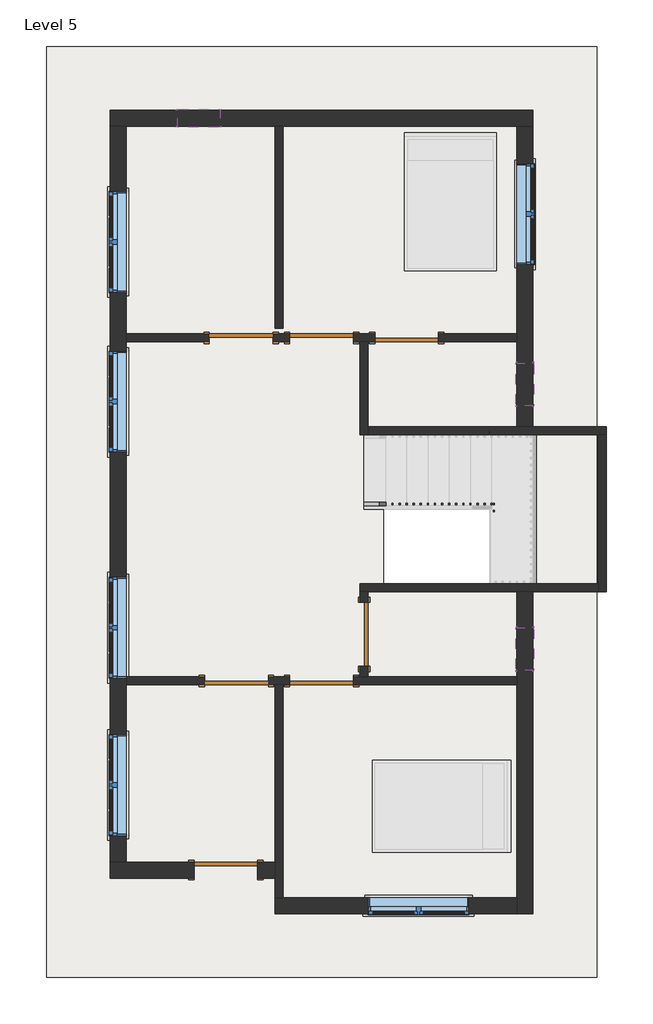
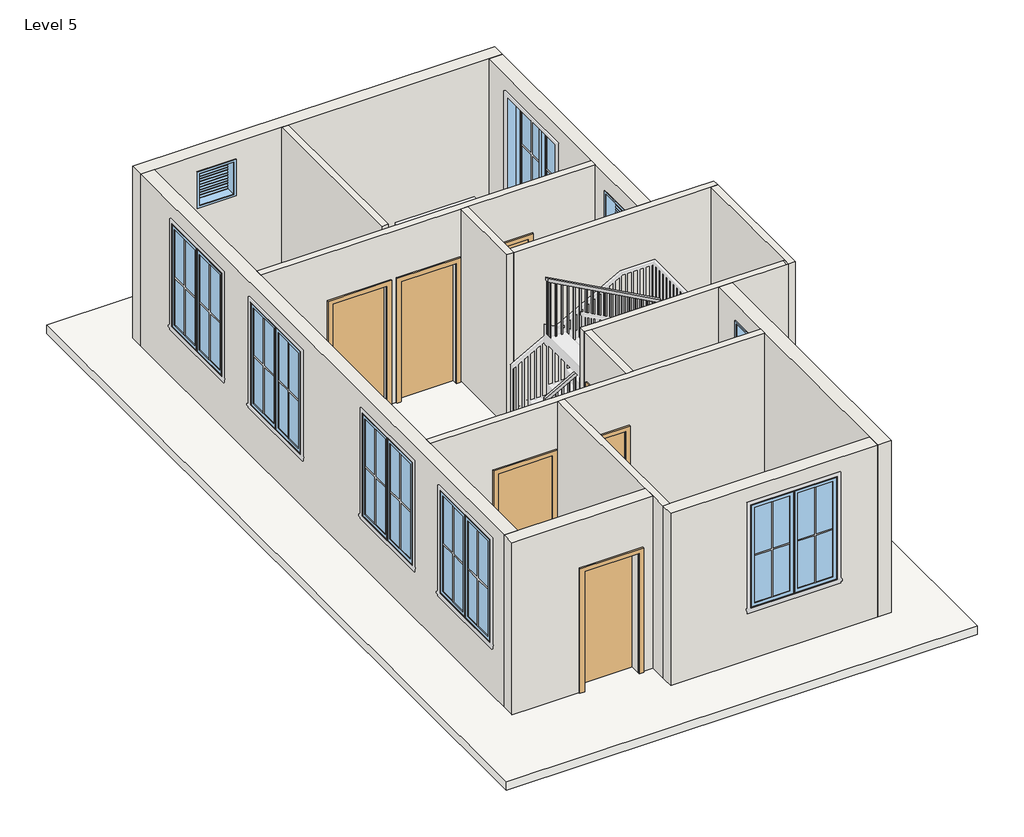
# One storey, part 1 of 2: 15 walls, 9 windows, 7 doors, 1 railing, 1 roof.
"""IFC4 building model written with IfcOpenShell, lengths in millimetres."""

from ifc_helpers import new_model, si_unit, frame, origin, place, context, project, spatial, polyline, outline, extrude, faceted_brep, transform, mapped, element, save
from components import door_e5f9f3c4, door_305aa2a5, door_0ca8825f, window_9ac97e1a, window_f2d8fef0

model = new_model("IFC4")

# Units and contexts
model_context = context("Model", 3, world=origin())
ifc_project = project(units=[si_unit("LENGTHUNIT", "METRE", prefix="MILLI")], contexts=[model_context])

# Site, building, storey
site = spatial("IfcSite", under=ifc_project)
building = spatial("IfcBuilding", under=site)
storey = spatial("IfcBuildingStorey", under=building, Name="Level 5", Elevation=9601.2)

# Doors
placement = place(None, origin())
door_shape = door_e5f9f3c4(model_context)
element("IfcDoor", 1, ObjectType="Single-Flush : 36\" x 84\"", at=placement, inside=storey, context=model_context, shape_type="MappedRepresentation", body=[
    mapped(door_shape, transform((-2929.7888307, 2238.9017201, 9601.2), x_axis=(1.0, 0.0, 0.0), y_axis=(0.0, 1.0, 0.0), z_axis=(0.0, 0.0, 1.0))),
])
element("IfcDoor", 2, ObjectType="Single-Flush : 36\" x 84\"", at=placement, inside=storey, context=model_context, shape_type="MappedRepresentation", body=[
    mapped(door_shape, transform((-558.0638307, 2238.9017201, 9601.2), x_axis=(-1.0, 0.0, 0.0), y_axis=(0.0, -1.0, 0.0), z_axis=(0.0, 0.0, 1.0))),
])
element("IfcDoor", 3, ObjectType="Single-Flush : 36\" x 84\"", at=placement, inside=storey, context=model_context, shape_type="MappedRepresentation", body=[
    mapped(door_shape, transform((-1167.6638307, -2009.2482799, 9601.2), x_axis=(0.0, -1.0, 0.0), y_axis=(1.0, 0.0, 0.0), z_axis=(0.0, 0.0, 1.0))),
])
element("IfcDoor", 4, ObjectType="Single-Flush : 36\" x 84\"", at=placement, inside=storey, context=model_context, shape_type="MappedRepresentation", body=[
    mapped(door_shape, transform((-1777.2638307, -2675.9982799, 9601.2), x_axis=(-1.0, 0.0, 0.0), y_axis=(0.0, -1.0, 0.0), z_axis=(0.0, 0.0, 1.0))),
])
door_2_shape = door_305aa2a5(model_context)
element("IfcDoor", 5, ObjectType="Single-Flush : 36\" x 84\"", at=placement, inside=storey, context=model_context, shape_type="MappedRepresentation", body=[
    mapped(door_2_shape, transform((-1777.2638307, 2238.9017201, 9601.2), x_axis=(-1.0, 0.0, 0.0), y_axis=(0.0, -1.0, 0.0), z_axis=(0.0, 0.0, 1.0))),
])
element("IfcDoor", 6, ObjectType="Single-Flush : 36\" x 84\"", at=placement, inside=storey, context=model_context, shape_type="MappedRepresentation", body=[
    mapped(door_2_shape, transform((-2996.4638307, -2675.9982799, 9601.2), x_axis=(1.0, 0.0, 0.0), y_axis=(0.0, 1.0, 0.0), z_axis=(0.0, 0.0, 1.0))),
])
door_3_shape = door_0ca8825f(model_context)
element("IfcDoor", 7, ObjectType="Single-Flush : 36\" x 84\"", at=placement, inside=storey, context=model_context, shape_type="MappedRepresentation", body=[
    mapped(door_3_shape, transform((-3148.8638307, -5387.4482799, 9601.2), x_axis=(1.0, 0.0, 0.0), y_axis=(0.0, 1.0, 0.0), z_axis=(0.0, 0.0, 1.0))),
])

# Railing
element("IfcRailing", 8, ObjectType="Handrail - Rectangular", at=placement, inside=storey, context=model_context, shape_type="SolidModel", body=[
    faceted_brep([(-1167.6638307, -116.9482799, 10684.9333333), (-1167.6638307, -116.9482799, 10626.8675836), (-1167.6638307, -167.7482799, 10626.8675836), (-1167.6638307, -167.7482799, 10684.9333333), (591.2861693, -116.9482799, 11658.7464821), (642.0861693, -116.9482799, 11628.8052998), (642.0861693, -167.7482799, 11628.8052998), (591.2861693, -167.7482799, 11658.7464821), (591.2861693, -116.9482799, 11700.9333333), (642.0861693, -116.9482799, 11650.1333333), (642.0861693, -167.7482799, 11650.1333333), (591.2861693, -167.7482799, 11700.9333333), (718.2861693, -116.9482799, 11700.9333333), (718.2861693, -116.9482799, 11650.1333333), (667.4861693, -167.7482799, 11650.1333333), (667.4861693, -167.7482799, 11700.9333333), (718.2861693, -218.5482799, 11700.9333333), (667.4861693, -218.5482799, 11700.9333333), (667.4861693, -269.3482799, 11650.1333333), (718.2861693, -269.3482799, 11650.1333333)], [[[0, 1, 2, 3]], [[1, 0, 4, 5]], [[2, 1, 5, 6]], [[3, 2, 6, 7]], [[0, 3, 7, 4]], [[5, 4, 8, 9]], [[6, 5, 9, 10]], [[7, 6, 10, 11]], [[4, 7, 11, 8]], [[9, 8, 12, 13]], [[10, 9, 13, 14]], [[11, 10, 14, 15]], [[8, 11, 15, 12]], [[16, 17, 18, 19]], [[13, 12, 16, 19]], [[14, 13, 19, 18]], [[15, 14, 18, 17]], [[12, 15, 17, 16]]]),
    faceted_brep([(718.2861693, -218.5482799, 11700.9333333), (718.2861693, -269.3482799, 11650.1333333), (667.4861693, -269.3482799, 11650.1333333), (667.4861693, -218.5482799, 11700.9333333), (718.2861693, -218.5482799, 11842.4310502), (667.4861693, -218.5482799, 11812.3403208), (667.4861693, -269.3482799, 11812.3403208), (718.2861693, -269.3482799, 11842.4310502)], [[[0, 1, 2, 3]], [[4, 5, 6, 7]], [[1, 0, 4, 7]], [[2, 1, 7, 6]], [[3, 2, 6, 5]], [[0, 3, 5, 4]]]),
    faceted_brep([(718.2861693, -269.3482799, 11842.4310502), (667.4861693, -269.3482799, 11812.3403208), (667.4861693, -218.5482799, 11812.3403208), (718.2861693, -218.5482799, 11842.4310502), (-1186.7138307, -269.3482799, 12886.2666667), (-1186.7138307, -218.5482799, 12886.2666667), (-1186.7138307, -218.5482799, 12828.3403208), (-1186.7138307, -269.3482799, 12828.3403208)], [[[0, 1, 2, 3]], [[4, 5, 6, 7]], [[1, 0, 4, 7]], [[2, 1, 7, 6]], [[3, 2, 6, 5]], [[0, 3, 5, 4]]]),
    extrude(outline(polyline([(12795.2855263, -1126.3888307), (12805.7238825, -1145.4388307), (11802.5333333, -1145.4388307), (11802.5333333, -1126.3888307), (12795.2855263, -1126.3888307)])), frame((0.0, -253.4732799, 0.0), z_axis=(0.0, 1.0, 0.0), x_axis=(0.0, 0.0, 1.0)), (0.0, 0.0, 1.0), 19.05),
    extrude(outline(polyline([(12739.6142934, -1024.7888307), (12750.0526496, -1043.8388307), (11802.5333333, -1043.8388307), (11802.5333333, -1024.7888307), (12739.6142934, -1024.7888307)])), frame((0.0, -253.4732799, 0.0), z_axis=(0.0, 1.0, 0.0), x_axis=(0.0, 0.0, 1.0)), (0.0, 0.0, 1.0), 19.05),
    extrude(outline(polyline([(12683.9430606, -923.1888307), (12694.3814167, -942.2388307), (11802.5333333, -942.2388307), (11802.5333333, -923.1888307), (12683.9430606, -923.1888307)])), frame((0.0, -253.4732799, 0.0), z_axis=(0.0, 1.0, 0.0), x_axis=(0.0, 0.0, 1.0)), (0.0, 0.0, 1.0), 19.05),
    extrude(outline(polyline([(12628.2718277, -821.5888307), (12638.7101838, -840.6388307), (11633.2, -840.6388307), (11633.2, -821.5888307), (12628.2718277, -821.5888307)])), frame((0.0, -253.4732799, 0.0), z_axis=(0.0, 1.0, 0.0), x_axis=(0.0, 0.0, 1.0)), (0.0, 0.0, 1.0), 19.05),
    extrude(outline(polyline([(12572.6005948, -719.9888307), (12583.038951, -739.0388307), (11633.2, -739.0388307), (11633.2, -719.9888307), (12572.6005948, -719.9888307)])), frame((0.0, -253.4732799, 0.0), z_axis=(0.0, 1.0, 0.0), x_axis=(0.0, 0.0, 1.0)), (0.0, 0.0, 1.0), 19.05),
    extrude(outline(polyline([(12516.9293619, -618.3888307), (12527.3677181, -637.4388307), (11633.2, -637.4388307), (11633.2, -618.3888307), (12516.9293619, -618.3888307)])), frame((0.0, -253.4732799, 0.0), z_axis=(0.0, 1.0, 0.0), x_axis=(0.0, 0.0, 1.0)), (0.0, 0.0, 1.0), 19.05),
    extrude(outline(polyline([(12461.258129, -516.7888307), (12471.6964852, -535.8388307), (11463.8666667, -535.8388307), (11463.8666667, -516.7888307), (12461.258129, -516.7888307)])), frame((0.0, -253.4732799, 0.0), z_axis=(0.0, 1.0, 0.0), x_axis=(0.0, 0.0, 1.0)), (0.0, 0.0, 1.0), 19.05),
    extrude(outline(polyline([(12405.5868962, -415.1888307), (12416.0252523, -434.2388307), (11463.8666667, -434.2388307), (11463.8666667, -415.1888307), (12405.5868962, -415.1888307)])), frame((0.0, -253.4732799, 0.0), z_axis=(0.0, 1.0, 0.0), x_axis=(0.0, 0.0, 1.0)), (0.0, 0.0, 1.0), 19.05),
    extrude(outline(polyline([(12349.9156633, -313.5888307), (12360.3540195, -332.6388307), (11463.8666667, -332.6388307), (11463.8666667, -313.5888307), (12349.9156633, -313.5888307)])), frame((0.0, -253.4732799, 0.0), z_axis=(0.0, 1.0, 0.0), x_axis=(0.0, 0.0, 1.0)), (0.0, 0.0, 1.0), 19.05),
    extrude(outline(polyline([(12294.2444304, -211.9888307), (12304.6827866, -231.0388307), (11294.5333333, -231.0388307), (11294.5333333, -211.9888307), (12294.2444304, -211.9888307)])), frame((0.0, -253.4732799, 0.0), z_axis=(0.0, 1.0, 0.0), x_axis=(0.0, 0.0, 1.0)), (0.0, 0.0, 1.0), 19.05),
    extrude(outline(polyline([(12238.5731975, -110.3888307), (12249.0115537, -129.4388307), (11294.5333333, -129.4388307), (11294.5333333, -110.3888307), (12238.5731975, -110.3888307)])), frame((0.0, -253.4732799, 0.0), z_axis=(0.0, 1.0, 0.0), x_axis=(0.0, 0.0, 1.0)), (0.0, 0.0, 1.0), 19.05),
    extrude(outline(polyline([(12182.9019647, -8.7888307), (12193.3403208, -27.8388307), (11294.5333333, -27.8388307), (11294.5333333, -8.7888307), (12182.9019647, -8.7888307)])), frame((0.0, -253.4732799, 0.0), z_axis=(0.0, 1.0, 0.0), x_axis=(0.0, 0.0, 1.0)), (0.0, 0.0, 1.0), 19.05),
    extrude(outline(polyline([(12127.2307318, 92.8111693), (12137.6690879, 73.7611693), (11125.2, 73.7611693), (11125.2, 92.8111693), (12127.2307318, 92.8111693)])), frame((0.0, -253.4732799, 0.0), z_axis=(0.0, 1.0, 0.0), x_axis=(0.0, 0.0, 1.0)), (0.0, 0.0, 1.0), 19.05),
    extrude(outline(polyline([(12071.5594989, 194.4111693), (12081.9978551, 175.3611693), (11125.2, 175.3611693), (11125.2, 194.4111693), (12071.5594989, 194.4111693)])), frame((0.0, -253.4732799, 0.0), z_axis=(0.0, 1.0, 0.0), x_axis=(0.0, 0.0, 1.0)), (0.0, 0.0, 1.0), 19.05),
    extrude(outline(polyline([(12015.888266, 296.0111693), (12026.3266222, 276.9611693), (11125.2, 276.9611693), (11125.2, 296.0111693), (12015.888266, 296.0111693)])), frame((0.0, -253.4732799, 0.0), z_axis=(0.0, 1.0, 0.0), x_axis=(0.0, 0.0, 1.0)), (0.0, 0.0, 1.0), 19.05),
    extrude(outline(polyline([(11960.2170332, 397.6111693), (11970.6553893, 378.5611693), (10955.8666667, 378.5611693), (10955.8666667, 397.6111693), (11960.2170332, 397.6111693)])), frame((0.0, -253.4732799, 0.0), z_axis=(0.0, 1.0, 0.0), x_axis=(0.0, 0.0, 1.0)), (0.0, 0.0, 1.0), 19.05),
    extrude(outline(polyline([(11904.5458003, 499.2111693), (11914.9841564, 480.1611693), (10955.8666667, 480.1611693), (10955.8666667, 499.2111693), (11904.5458003, 499.2111693)])), frame((0.0, -253.4732799, 0.0), z_axis=(0.0, 1.0, 0.0), x_axis=(0.0, 0.0, 1.0)), (0.0, 0.0, 1.0), 19.05),
    extrude(outline(polyline([(11848.8745674, 600.8111693), (11859.3129236, 581.7611693), (10955.8666667, 581.7611693), (10955.8666667, 600.8111693), (11848.8745674, 600.8111693)])), frame((0.0, -253.4732799, 0.0), z_axis=(0.0, 1.0, 0.0), x_axis=(0.0, 0.0, 1.0)), (0.0, 0.0, 1.0), 19.05),
    extrude(outline(polyline([(651.6111693, -151.8732799), (651.6111693, -132.8232799), (670.6611693, -132.8232799), (670.6611693, -151.8732799), (651.6111693, -151.8732799)])), frame((0.0, 0.0, 10617.2), z_axis=(0.0, 0.0, 1.0), x_axis=(1.0, 0.0, 0.0)), (0.0, 0.0, 1.0), 1032.9333333),
    extrude(outline(polyline([(11588.3762341, 569.0611693), (11577.8295213, 550.0111693), (10617.2, 550.0111693), (10617.2, 569.0611693), (11588.3762341, 569.0611693)])), frame((0.0, -151.8732799, 0.0), z_axis=(0.0, 1.0, 0.0), x_axis=(0.0, 0.0, 1.0)), (0.0, 0.0, 1.0), 19.05),
    extrude(outline(polyline([(11532.1270991, 467.4611693), (11521.5803863, 448.4111693), (10617.2, 448.4111693), (10617.2, 467.4611693), (11532.1270991, 467.4611693)])), frame((0.0, -151.8732799, 0.0), z_axis=(0.0, 1.0, 0.0), x_axis=(0.0, 0.0, 1.0)), (0.0, 0.0, 1.0), 19.05),
    extrude(outline(polyline([(11475.8779642, 365.8611693), (11465.3312514, 346.8111693), (10447.8666667, 346.8111693), (10447.8666667, 365.8611693), (11475.8779642, 365.8611693)])), frame((0.0, -151.8732799, 0.0), z_axis=(0.0, 1.0, 0.0), x_axis=(0.0, 0.0, 1.0)), (0.0, 0.0, 1.0), 19.05),
    extrude(outline(polyline([(11419.6288292, 264.2611693), (11409.0821164, 245.2111693), (10447.8666667, 245.2111693), (10447.8666667, 264.2611693), (11419.6288292, 264.2611693)])), frame((0.0, -151.8732799, 0.0), z_axis=(0.0, 1.0, 0.0), x_axis=(0.0, 0.0, 1.0)), (0.0, 0.0, 1.0), 19.05),
    extrude(outline(polyline([(11363.3796943, 162.6611693), (11352.8329815, 143.6111693), (10447.8666667, 143.6111693), (10447.8666667, 162.6611693), (11363.3796943, 162.6611693)])), frame((0.0, -151.8732799, 0.0), z_axis=(0.0, 1.0, 0.0), x_axis=(0.0, 0.0, 1.0)), (0.0, 0.0, 1.0), 19.05),
    extrude(outline(polyline([(11307.1305593, 61.0611693), (11296.5838465, 42.0111693), (10278.5333333, 42.0111693), (10278.5333333, 61.0611693), (11307.1305593, 61.0611693)])), frame((0.0, -151.8732799, 0.0), z_axis=(0.0, 1.0, 0.0), x_axis=(0.0, 0.0, 1.0)), (0.0, 0.0, 1.0), 19.05),
    extrude(outline(polyline([(11250.8814244, -40.5388307), (11240.3347116, -59.5888307), (10278.5333333, -59.5888307), (10278.5333333, -40.5388307), (11250.8814244, -40.5388307)])), frame((0.0, -151.8732799, 0.0), z_axis=(0.0, 1.0, 0.0), x_axis=(0.0, 0.0, 1.0)), (0.0, 0.0, 1.0), 19.05),
    extrude(outline(polyline([(11194.6322895, -142.1388307), (11184.0855766, -161.1888307), (10278.5333333, -161.1888307), (10278.5333333, -142.1388307), (11194.6322895, -142.1388307)])), frame((0.0, -151.8732799, 0.0), z_axis=(0.0, 1.0, 0.0), x_axis=(0.0, 0.0, 1.0)), (0.0, 0.0, 1.0), 19.05),
    extrude(outline(polyline([(11138.3831545, -243.7388307), (11127.8364417, -262.7888307), (10109.2, -262.7888307), (10109.2, -243.7388307), (11138.3831545, -243.7388307)])), frame((0.0, -151.8732799, 0.0), z_axis=(0.0, 1.0, 0.0), x_axis=(0.0, 0.0, 1.0)), (0.0, 0.0, 1.0), 19.05),
    extrude(outline(polyline([(11082.1340196, -345.3388307), (11071.5873068, -364.3888307), (10109.2, -364.3888307), (10109.2, -345.3388307), (11082.1340196, -345.3388307)])), frame((0.0, -151.8732799, 0.0), z_axis=(0.0, 1.0, 0.0), x_axis=(0.0, 0.0, 1.0)), (0.0, 0.0, 1.0), 19.05),
    extrude(outline(polyline([(11025.8848846, -446.9388307), (11015.3381718, -465.9888307), (10109.2, -465.9888307), (10109.2, -446.9388307), (11025.8848846, -446.9388307)])), frame((0.0, -151.8732799, 0.0), z_axis=(0.0, 1.0, 0.0), x_axis=(0.0, 0.0, 1.0)), (0.0, 0.0, 1.0), 19.05),
    extrude(outline(polyline([(10969.6357497, -548.5388307), (10959.0890369, -567.5888307), (9939.8666667, -567.5888307), (9939.8666667, -548.5388307), (10969.6357497, -548.5388307)])), frame((0.0, -151.8732799, 0.0), z_axis=(0.0, 1.0, 0.0), x_axis=(0.0, 0.0, 1.0)), (0.0, 0.0, 1.0), 19.05),
    extrude(outline(polyline([(10913.3866147, -650.1388307), (10902.8399019, -669.1888307), (9939.8666667, -669.1888307), (9939.8666667, -650.1388307), (10913.3866147, -650.1388307)])), frame((0.0, -151.8732799, 0.0), z_axis=(0.0, 1.0, 0.0), x_axis=(0.0, 0.0, 1.0)), (0.0, 0.0, 1.0), 19.05),
    extrude(outline(polyline([(10857.1374798, -751.7388307), (10846.590767, -770.7888307), (9939.8666667, -770.7888307), (9939.8666667, -751.7388307), (10857.1374798, -751.7388307)])), frame((0.0, -151.8732799, 0.0), z_axis=(0.0, 1.0, 0.0), x_axis=(0.0, 0.0, 1.0)), (0.0, 0.0, 1.0), 19.05),
    extrude(outline(polyline([(10800.8883448, -853.3388307), (10790.341632, -872.3888307), (9770.5333333, -872.3888307), (9770.5333333, -853.3388307), (10800.8883448, -853.3388307)])), frame((0.0, -151.8732799, 0.0), z_axis=(0.0, 1.0, 0.0), x_axis=(0.0, 0.0, 1.0)), (0.0, 0.0, 1.0), 19.05),
    extrude(outline(polyline([(10744.6392099, -954.9388307), (10734.0924971, -973.9888307), (9770.5333333, -973.9888307), (9770.5333333, -954.9388307), (10744.6392099, -954.9388307)])), frame((0.0, -151.8732799, 0.0), z_axis=(0.0, 1.0, 0.0), x_axis=(0.0, 0.0, 1.0)), (0.0, 0.0, 1.0), 19.05),
    extrude(outline(polyline([(10688.3900749, -1056.5388307), (10677.8433621, -1075.5888307), (9770.5333333, -1075.5888307), (9770.5333333, -1056.5388307), (10688.3900749, -1056.5388307)])), frame((0.0, -151.8732799, 0.0), z_axis=(0.0, 1.0, 0.0), x_axis=(0.0, 0.0, 1.0)), (0.0, 0.0, 1.0), 19.05),
    extrude(outline(polyline([(683.3611693, -234.4232799), (702.4111693, -234.4232799), (702.4111693, -253.4732799), (683.3611693, -253.4732799), (683.3611693, -234.4232799)])), frame((0.0, 0.0, 10786.5333333), z_axis=(0.0, 0.0, 1.0), x_axis=(1.0, 0.0, 0.0)), (0.0, 0.0, 1.0), 863.6),
    extrude(outline(polyline([(683.3611693, -151.8732799), (683.3611693, -132.8232799), (702.4111693, -132.8232799), (702.4111693, -151.8732799), (683.3611693, -151.8732799)])), frame((0.0, 0.0, 10786.5333333), z_axis=(0.0, 0.0, 1.0), x_axis=(1.0, 0.0, 0.0)), (0.0, 0.0, 1.0), 863.6),
    extrude(outline(polyline([(12817.9019647, -1167.6638307), (12828.3403208, -1186.7138307), (11802.5333333, -1186.7138307), (11802.5333333, -1167.6638307), (12817.9019647, -1167.6638307)])), frame((0.0, -253.4732799, 0.0), z_axis=(0.0, 1.0, 0.0), x_axis=(0.0, 0.0, 1.0)), (0.0, 0.0, 1.0), 19.05),
    extrude(outline(polyline([(10637.4142964, -1148.6138307), (10626.8675836, -1167.6638307), (9770.5333333, -1167.6638307), (9770.5333333, -1148.6138307), (10637.4142964, -1148.6138307)])), frame((0.0, -151.8732799, 0.0), z_axis=(0.0, 1.0, 0.0), x_axis=(0.0, 0.0, 1.0)), (0.0, 0.0, 1.0), 19.05),
])

# Roof
element("IfcRoof", 9, ObjectType="ROOF 6\"", at=placement, inside=storey, context=model_context, shape_type="SweptSolid", body=[
    extrude(outline(polyline([(-5720.6138307, -6924.1482799), (-5720.6138307, 6410.8517201), (2166.0861693, 6410.8517201), (2166.0861693, -6924.1482799), (-5720.6138307, -6924.1482799)]), holes=[polyline([(1251.6861693, -1285.3482799), (1251.6861693, 899.0517201), (-881.9138307, 899.0517201), (-881.9138307, -1285.3482799), (1251.6861693, -1285.3482799)])]), frame((0.0, 0.0, 9448.8), z_axis=(0.0, 0.0, 1.0), x_axis=(1.0, 0.0, 0.0)), (0.0, 0.0, 1.0), 152.4),
])

# Walls
element("IfcWall", 10, ObjectType="WALL 4.5\"", at=placement, inside=storey, context=model_context, shape_type="SweptSolid", body=[
    extrude(outline(polyline([(-2444.0138307, 2372.2517201), (-2444.0138307, 5267.8517201), (-2329.7138307, 5267.8517201), (-2329.7138307, 2372.2517201), (-2444.0138307, 2372.2517201)])), frame((0.0, 0.0, 9601.2), z_axis=(0.0, 0.0, 1.0), x_axis=(1.0, 0.0, 0.0)), (0.0, 0.0, 1.0), 3048.0),
])
element("IfcWall", 11, ObjectType="WALL 4.5\"", at=placement, inside=storey, context=model_context, shape_type="Brep", body=[
    faceted_brep([(-1320.0638307, 2181.7517201, 9601.2), (-1224.8138307, 2181.7517201, 9601.2), (-1110.5138307, 2181.7517201, 9601.2), (-1015.2638307, 2181.7517201, 9601.2), (-1015.2638307, 2181.7517201, 11734.8), (-100.8638307, 2181.7517201, 11734.8), (-100.8638307, 2181.7517201, 9601.2), (1023.0861693, 2181.7517201, 9601.2), (1023.0861693, 2181.7517201, 12649.2), (-1110.5138307, 2181.7517201, 12649.2), (-1224.8138307, 2181.7517201, 12649.2), (-4577.6138307, 2181.7517201, 12649.2), (-4577.6138307, 2181.7517201, 9601.2), (-3386.9888307, 2181.7517201, 9601.2), (-3386.9888307, 2181.7517201, 11734.8), (-2472.5888307, 2181.7517201, 11734.8), (-2472.5888307, 2181.7517201, 9601.2), (-2234.4638307, 2181.7517201, 9601.2), (-2234.4638307, 2181.7517201, 11734.8), (-1320.0638307, 2181.7517201, 11734.8), (-1015.2638307, 2296.0517201, 11734.8), (-1015.2638307, 2296.0517201, 9601.2), (-1320.0638307, 2296.0517201, 9601.2), (-1320.0638307, 2296.0517201, 11734.8), (-2234.4638307, 2296.0517201, 11734.8), (-2234.4638307, 2296.0517201, 9601.2), (-2472.5888307, 2296.0517201, 9601.2), (-2472.5888307, 2296.0517201, 11734.8), (-3386.9888307, 2296.0517201, 11734.8), (-3386.9888307, 2296.0517201, 9601.2), (-4577.6138307, 2296.0517201, 9601.2), (-4577.6138307, 2296.0517201, 12649.2), (1023.0861693, 2296.0517201, 12649.2), (1023.0861693, 2296.0517201, 9601.2), (-100.8638307, 2296.0517201, 9601.2), (-100.8638307, 2296.0517201, 11734.8)], [[[0, 1, 2, 3, 4, 5, 6, 7, 8, 9, 10, 11, 12, 13, 14, 15, 16, 17, 18, 19]], [[20, 21, 22, 23, 24, 25, 26, 27, 28, 29, 30, 31, 32, 33, 34, 35]], [[13, 12, 30, 29]], [[26, 25, 17, 16]], [[34, 33, 7, 6]], [[22, 21, 3, 2, 1, 0]], [[8, 7, 33, 32]], [[12, 11, 31, 30]], [[27, 26, 16, 15]], [[28, 27, 15, 14]], [[29, 28, 14, 13]], [[18, 17, 25, 24]], [[19, 18, 24, 23]], [[0, 19, 23, 22]], [[4, 3, 21, 20]], [[5, 4, 20, 35]], [[6, 5, 35, 34]], [[11, 10, 9, 8, 32, 31]]]),
])
element("IfcWall", 12, ObjectType="WALL 4.5\"", at=placement, inside=storey, context=model_context, shape_type="Brep", body=[
    faceted_brep([(-1224.8138307, 2181.7517201, 9601.2), (-1224.8138307, 848.2517201, 9601.2), (-1224.8138307, 848.2517201, 12649.2), (-1224.8138307, 2181.7517201, 12649.2), (-1110.5138307, 2181.7517201, 9601.2), (-1110.5138307, 2181.7517201, 12649.2), (-1110.5138307, 962.5517201, 12649.2), (-1110.5138307, 848.2517201, 12649.2), (-1110.5138307, 848.2517201, 9601.2), (-1110.5138307, 962.5517201, 9601.2)], [[[0, 1, 2, 3]], [[4, 5, 6, 7, 8, 9]], [[1, 0, 4, 9, 8]], [[0, 3, 5, 4]], [[2, 1, 8, 7]], [[3, 2, 7, 6, 5]]]),
])
element("IfcWall", 13, ObjectType="WALL 4.5\"", at=placement, inside=storey, context=model_context, shape_type="Brep", body=[
    faceted_brep([(-1110.5138307, 848.2517201, 9601.2), (2191.4861693, 848.2517201, 9601.2), (2305.7861693, 848.2517201, 9601.2), (2305.7861693, 848.2517201, 12649.2), (2191.4861693, 848.2517201, 12649.2), (-1110.5138307, 848.2517201, 12649.2), (-1110.5138307, 962.5517201, 9601.2), (-1110.5138307, 962.5517201, 12649.2), (1023.0861693, 962.5517201, 12649.2), (1251.6861693, 962.5517201, 12649.2), (2305.7861693, 962.5517201, 12649.2), (2305.7861693, 962.5517201, 9601.2), (1251.6861693, 962.5517201, 9601.2), (1023.0861693, 962.5517201, 9601.2)], [[[0, 1, 2, 3, 4, 5]], [[6, 7, 8, 9, 10, 11, 12, 13]], [[2, 1, 0, 6, 13, 12, 11]], [[5, 4, 3, 10, 9, 8, 7]], [[0, 5, 7, 6]], [[3, 2, 11, 10]]]),
])
element("IfcWall", 14, ObjectType="WALL 4.5\"", at=placement, inside=storey, context=model_context, shape_type="Brep", body=[
    faceted_brep([(2191.4861693, 848.2517201, 9601.2), (2191.4861693, -1285.3482799, 9601.2), (2191.4861693, -1399.6482799, 9601.2), (2191.4861693, -1399.6482799, 12649.2), (2191.4861693, -1285.3482799, 12649.2), (2191.4861693, 848.2517201, 12649.2), (2305.7861693, 848.2517201, 9601.2), (2305.7861693, 848.2517201, 12649.2), (2305.7861693, -1399.6482799, 12649.2), (2305.7861693, -1399.6482799, 9601.2)], [[[0, 1, 2, 3, 4, 5]], [[6, 7, 8, 9]], [[2, 1, 0, 6, 9]], [[5, 4, 3, 8, 7]], [[0, 5, 7, 6]], [[3, 2, 9, 8]]]),
])
element("IfcWall", 15, ObjectType="WALL 4.5\"", at=placement, inside=storey, context=model_context, shape_type="Brep", body=[
    faceted_brep([(2191.4861693, -1285.3482799, 9601.2), (-1224.8138307, -1285.3482799, 9601.2), (-1224.8138307, -1285.3482799, 12649.2), (-881.9138307, -1285.3482799, 12649.2), (1251.6861693, -1285.3482799, 12649.2), (2166.0861693, -1285.3482799, 12649.2), (2191.4861693, -1285.3482799, 12649.2), (2191.4861693, -1399.6482799, 9601.2), (2191.4861693, -1399.6482799, 12649.2), (2166.0861693, -1399.6482799, 12649.2), (1251.6861693, -1399.6482799, 12649.2), (1023.0861693, -1399.6482799, 12649.2), (-1110.5138307, -1399.6482799, 12649.2), (-1224.8138307, -1399.6482799, 12649.2), (-1224.8138307, -1399.6482799, 9601.2), (-1110.5138307, -1399.6482799, 9601.2), (1023.0861693, -1399.6482799, 9601.2), (1251.6861693, -1399.6482799, 9601.2)], [[[0, 1, 2, 3, 4, 5, 6]], [[7, 8, 9, 10, 11, 12, 13, 14, 15, 16, 17]], [[1, 0, 7, 17, 16, 15, 14]], [[0, 6, 8, 7]], [[2, 1, 14, 13]], [[6, 5, 9, 8]], [[5, 4, 3, 2, 13, 12, 11, 10, 9]]]),
])
element("IfcWall", 16, ObjectType="WALL 4.5\"", at=placement, inside=storey, context=model_context, shape_type="SweptSolid", body=[
    extrude(outline(polyline([(-2466.4482799, 11734.8), (-2466.4482799, 9601.2), (-2618.8482799, 9601.2), (-2618.8482799, 12649.2), (-1399.6482799, 12649.2), (-1399.6482799, 9601.2), (-1552.0482799, 9601.2), (-1552.0482799, 11734.8), (-2466.4482799, 11734.8)])), frame((-1224.8138307, 0.0, 0.0), z_axis=(1.0, 0.0, 0.0), x_axis=(0.0, 1.0, 0.0)), (0.0, 0.0, 1.0), 114.3),
])
element("IfcWall", 17, ObjectType="WALL 4.5\"", at=placement, inside=storey, context=model_context, shape_type="Brep", body=[
    faceted_brep([(-2234.4638307, -2618.8482799, 9601.2), (-2539.2638307, -2618.8482799, 9601.2), (-2539.2638307, -2618.8482799, 11734.8), (-3453.6638307, -2618.8482799, 11734.8), (-3453.6638307, -2618.8482799, 9601.2), (-4577.6138307, -2618.8482799, 9601.2), (-4577.6138307, -2618.8482799, 12649.2), (-1224.8138307, -2618.8482799, 12649.2), (-1110.5138307, -2618.8482799, 12649.2), (1023.0861693, -2618.8482799, 12649.2), (1023.0861693, -2618.8482799, 9601.2), (-1110.5138307, -2618.8482799, 9601.2), (-1224.8138307, -2618.8482799, 9601.2), (-1320.0638307, -2618.8482799, 9601.2), (-1320.0638307, -2618.8482799, 11734.8), (-2234.4638307, -2618.8482799, 11734.8), (-2539.2638307, -2733.1482799, 11734.8), (-2539.2638307, -2733.1482799, 9601.2), (-2444.0138307, -2733.1482799, 9601.2), (-2329.7138307, -2733.1482799, 9601.2), (-2234.4638307, -2733.1482799, 9601.2), (-2234.4638307, -2733.1482799, 11734.8), (-1320.0638307, -2733.1482799, 11734.8), (-1320.0638307, -2733.1482799, 9601.2), (1023.0861693, -2733.1482799, 9601.2), (1023.0861693, -2733.1482799, 12649.2), (-2329.7138307, -2733.1482799, 12649.2), (-2444.0138307, -2733.1482799, 12649.2), (-4577.6138307, -2733.1482799, 12649.2), (-4577.6138307, -2733.1482799, 9601.2), (-3453.6638307, -2733.1482799, 9601.2), (-3453.6638307, -2733.1482799, 11734.8)], [[[0, 1, 2, 3, 4, 5, 6, 7, 8, 9, 10, 11, 12, 13, 14, 15]], [[16, 17, 18, 19, 20, 21, 22, 23, 24, 25, 26, 27, 28, 29, 30, 31]], [[13, 12, 11, 10, 24, 23]], [[30, 29, 5, 4]], [[20, 19, 18, 17, 1, 0]], [[10, 9, 25, 24]], [[6, 5, 29, 28]], [[21, 20, 0, 15]], [[22, 21, 15, 14]], [[23, 22, 14, 13]], [[2, 1, 17, 16]], [[3, 2, 16, 31]], [[4, 3, 31, 30]], [[9, 8, 7, 6, 28, 27, 26, 25]]]),
])
element("IfcWall", 18, ObjectType="WALL 4.5\"", at=placement, inside=storey, context=model_context, shape_type="Brep", body=[
    faceted_brep([(-2329.7138307, -5781.1482799, 9601.2), (-2329.7138307, -2733.1482799, 9601.2), (-2329.7138307, -2733.1482799, 12649.2), (-2329.7138307, -5781.1482799, 12649.2), (-2444.0138307, -5781.1482799, 9601.2), (-2444.0138307, -5781.1482799, 12649.2), (-2444.0138307, -5501.7482799, 12649.2), (-2444.0138307, -5273.1482799, 12649.2), (-2444.0138307, -2733.1482799, 12649.2), (-2444.0138307, -2733.1482799, 9601.2), (-2444.0138307, -5273.1482799, 9601.2), (-2444.0138307, -5501.7482799, 9601.2)], [[[0, 1, 2, 3]], [[4, 5, 6, 7, 8, 9, 10, 11]], [[1, 0, 4, 11, 10, 9]], [[0, 3, 5, 4]], [[2, 1, 9, 8]], [[3, 2, 8, 7, 6, 5]]]),
])
element("IfcWall", 19, ObjectType="WALL 9\"", at=placement, inside=storey, context=model_context, shape_type="Brep", body=[
    faceted_brep([(-4806.2138307, 5267.8517201, 9601.2), (-4577.6138307, 5267.8517201, 9601.2), (-2444.0138307, 5267.8517201, 9601.2), (-2329.7138307, 5267.8517201, 9601.2), (1023.0861693, 5267.8517201, 9601.2), (1251.6861693, 5267.8517201, 9601.2), (1251.6861693, 5267.8517201, 12649.2), (1023.0861693, 5267.8517201, 12649.2), (-2329.7138307, 5267.8517201, 12649.2), (-2444.0138307, 5267.8517201, 12649.2), (-4577.6138307, 5267.8517201, 12649.2), (-4806.2138307, 5267.8517201, 12649.2), (-3844.1888307, 5267.8517201, 12344.4), (-3234.5888307, 5267.8517201, 12344.4), (-3234.5888307, 5267.8517201, 11734.8), (-3844.1888307, 5267.8517201, 11734.8), (-4806.2138307, 5496.4517201, 9601.2), (-4806.2138307, 5496.4517201, 12649.2), (1251.6861693, 5496.4517201, 12649.2), (1251.6861693, 5496.4517201, 9601.2), (-3844.1888307, 5496.4517201, 12344.4), (-3844.1888307, 5496.4517201, 11734.8), (-3234.5888307, 5496.4517201, 11734.8), (-3234.5888307, 5496.4517201, 12344.4)], [[[0, 1, 2, 3, 4, 5, 6, 7, 8, 9, 10, 11], [12, 13, 14, 15]], [[16, 17, 18, 19], [20, 21, 22, 23]], [[5, 4, 3, 2, 1, 0, 16, 19]], [[6, 5, 19, 18]], [[0, 11, 17, 16]], [[21, 20, 12, 15]], [[22, 21, 15, 14]], [[23, 22, 14, 13]], [[20, 23, 13, 12]], [[11, 10, 9, 8, 7, 6, 18, 17]]]),
])
element("IfcWall", 20, ObjectType="WALL 9\"", at=placement, inside=storey, context=model_context, shape_type="Brep", body=[
    faceted_brep([(1023.0861693, 5267.8517201, 9601.2), (1023.0861693, 2296.0517201, 9601.2), (1023.0861693, 2181.7517201, 9601.2), (1023.0861693, 962.5517201, 9601.2), (1023.0861693, 962.5517201, 12649.2), (1023.0861693, 2181.7517201, 12649.2), (1023.0861693, 2296.0517201, 12649.2), (1023.0861693, 5267.8517201, 12649.2), (1023.0861693, 3286.6517201, 12344.4), (1023.0861693, 3286.6517201, 10515.6), (1023.0861693, 4734.4517201, 10515.6), (1023.0861693, 4734.4517201, 12344.4), (1023.0861693, 1876.9517201, 12344.4), (1023.0861693, 1267.3517201, 12344.4), (1023.0861693, 1267.3517201, 11734.8), (1023.0861693, 1876.9517201, 11734.8), (1251.6861693, 5267.8517201, 9601.2), (1251.6861693, 5267.8517201, 12649.2), (1251.6861693, 962.5517201, 12649.2), (1251.6861693, 962.5517201, 9601.2), (1251.6861693, 3286.6517201, 12344.4), (1251.6861693, 4734.4517201, 12344.4), (1251.6861693, 4734.4517201, 10515.6), (1251.6861693, 3286.6517201, 10515.6), (1251.6861693, 1876.9517201, 12344.4), (1251.6861693, 1876.9517201, 11734.8), (1251.6861693, 1267.3517201, 11734.8), (1251.6861693, 1267.3517201, 12344.4)], [[[0, 1, 2, 3, 4, 5, 6, 7], [8, 9, 10, 11], [12, 13, 14, 15]], [[16, 17, 18, 19], [20, 21, 22, 23], [24, 25, 26, 27]], [[3, 2, 1, 0, 16, 19]], [[0, 7, 17, 16]], [[4, 3, 19, 18]], [[9, 8, 20, 23]], [[10, 9, 23, 22]], [[11, 10, 22, 21]], [[8, 11, 21, 20]], [[25, 24, 12, 15]], [[26, 25, 15, 14]], [[27, 26, 14, 13]], [[24, 27, 13, 12]], [[7, 6, 5, 4, 18, 17]]]),
])
element("IfcWall", 21, ObjectType="WALL 9\"", at=placement, inside=storey, context=model_context, shape_type="Brep", body=[
    faceted_brep([(1023.0861693, -1399.6482799, 9601.2), (1023.0861693, -2618.8482799, 9601.2), (1023.0861693, -2733.1482799, 9601.2), (1023.0861693, -5781.1482799, 9601.2), (1023.0861693, -6009.7482799, 9601.2), (1023.0861693, -6009.7482799, 12649.2), (1023.0861693, -5781.1482799, 12649.2), (1023.0861693, -2733.1482799, 12649.2), (1023.0861693, -2618.8482799, 12649.2), (1023.0861693, -1399.6482799, 12649.2), (1023.0861693, -1913.9982799, 12344.4), (1023.0861693, -2523.5982799, 12344.4), (1023.0861693, -2523.5982799, 11734.8), (1023.0861693, -1913.9982799, 11734.8), (1251.6861693, -1399.6482799, 9601.2), (1251.6861693, -1399.6482799, 12649.2), (1251.6861693, -6009.7482799, 12649.2), (1251.6861693, -6009.7482799, 9601.2), (1251.6861693, -1913.9982799, 12344.4), (1251.6861693, -1913.9982799, 11734.8), (1251.6861693, -2523.5982799, 11734.8), (1251.6861693, -2523.5982799, 12344.4)], [[[0, 1, 2, 3, 4, 5, 6, 7, 8, 9], [10, 11, 12, 13]], [[14, 15, 16, 17], [18, 19, 20, 21]], [[4, 3, 2, 1, 0, 14, 17]], [[5, 4, 17, 16]], [[0, 9, 15, 14]], [[19, 18, 10, 13]], [[20, 19, 13, 12]], [[21, 20, 12, 11]], [[18, 21, 11, 10]], [[9, 8, 7, 6, 5, 16, 15]]]),
])
element("IfcWall", 22, ObjectType="WALL 9\"", at=placement, inside=storey, context=model_context, shape_type="Brep", body=[
    faceted_brep([(1023.0861693, -5781.1482799, 9601.2), (-2329.7138307, -5781.1482799, 9601.2), (-2444.0138307, -5781.1482799, 9601.2), (-2444.0138307, -5781.1482799, 12649.2), (-2329.7138307, -5781.1482799, 12649.2), (1023.0861693, -5781.1482799, 12649.2), (-1110.5138307, -5781.1482799, 12344.4), (-1110.5138307, -5781.1482799, 10515.6), (337.2861693, -5781.1482799, 10515.6), (337.2861693, -5781.1482799, 12344.4), (1023.0861693, -6009.7482799, 9601.2), (1023.0861693, -6009.7482799, 12649.2), (-2444.0138307, -6009.7482799, 12649.2), (-2444.0138307, -6009.7482799, 9601.2), (-1110.5138307, -6009.7482799, 12344.4), (337.2861693, -6009.7482799, 12344.4), (337.2861693, -6009.7482799, 10515.6), (-1110.5138307, -6009.7482799, 10515.6)], [[[0, 1, 2, 3, 4, 5], [6, 7, 8, 9]], [[10, 11, 12, 13], [14, 15, 16, 17]], [[2, 1, 0, 10, 13]], [[0, 5, 11, 10]], [[3, 2, 13, 12]], [[7, 6, 14, 17]], [[8, 7, 17, 16]], [[9, 8, 16, 15]], [[6, 9, 15, 14]], [[5, 4, 3, 12, 11]]]),
])
element("IfcWall", 23, ObjectType="WALL 9\"", at=placement, inside=storey, context=model_context, shape_type="Brep", body=[
    faceted_brep([(-2691.6638307, -5501.7482799, 11734.8), (-2691.6638307, -5501.7482799, 9601.2), (-2444.0138307, -5501.7482799, 9601.2), (-2444.0138307, -5501.7482799, 12649.2), (-4806.2138307, -5501.7482799, 12649.2), (-4806.2138307, -5501.7482799, 9601.2), (-3606.0638307, -5501.7482799, 9601.2), (-3606.0638307, -5501.7482799, 11734.8), (-2444.0138307, -5273.1482799, 9601.2), (-2691.6638307, -5273.1482799, 9601.2), (-2691.6638307, -5273.1482799, 11734.8), (-3606.0638307, -5273.1482799, 11734.8), (-3606.0638307, -5273.1482799, 9601.2), (-4577.6138307, -5273.1482799, 9601.2), (-4806.2138307, -5273.1482799, 9601.2), (-4806.2138307, -5273.1482799, 12649.2), (-4577.6138307, -5273.1482799, 12649.2), (-2444.0138307, -5273.1482799, 12649.2)], [[[0, 1, 2, 3, 4, 5, 6, 7]], [[8, 9, 10, 11, 12, 13, 14, 15, 16, 17]], [[6, 5, 14, 13, 12]], [[2, 1, 9, 8]], [[5, 4, 15, 14]], [[3, 2, 8, 17]], [[10, 9, 1, 0]], [[11, 10, 0, 7]], [[12, 11, 7, 6]], [[4, 3, 17, 16, 15]]]),
])
element("IfcWall", 24, ObjectType="WALL 9\"", at=placement, inside=storey, context=model_context, shape_type="Brep", body=[
    faceted_brep([(-4577.6138307, -5273.1482799, 9601.2), (-4577.6138307, -2733.1482799, 9601.2), (-4577.6138307, -2618.8482799, 9601.2), (-4577.6138307, 2181.7517201, 9601.2), (-4577.6138307, 2296.0517201, 9601.2), (-4577.6138307, 5267.8517201, 9601.2), (-4577.6138307, 5267.8517201, 12649.2), (-4577.6138307, 2296.0517201, 12649.2), (-4577.6138307, 2181.7517201, 12649.2), (-4577.6138307, -2618.8482799, 12649.2), (-4577.6138307, -2733.1482799, 12649.2), (-4577.6138307, -5273.1482799, 12649.2), (-4577.6138307, -3444.3482799, 12344.4), (-4577.6138307, -3444.3482799, 10515.6), (-4577.6138307, -4892.1482799, 10515.6), (-4577.6138307, -4892.1482799, 12344.4), (-4577.6138307, -1190.0982799, 12344.4), (-4577.6138307, -1190.0982799, 10515.6), (-4577.6138307, -2637.8982799, 10515.6), (-4577.6138307, -2637.8982799, 12344.4), (-4577.6138307, 4334.4017201, 12344.4), (-4577.6138307, 4334.4017201, 10515.6), (-4577.6138307, 2886.6017201, 10515.6), (-4577.6138307, 2886.6017201, 12344.4), (-4577.6138307, 2048.4017201, 12344.4), (-4577.6138307, 2048.4017201, 10515.6), (-4577.6138307, 600.6017201, 10515.6), (-4577.6138307, 600.6017201, 12344.4), (-4806.2138307, -5273.1482799, 9601.2), (-4806.2138307, -5273.1482799, 12649.2), (-4806.2138307, 5267.8517201, 12649.2), (-4806.2138307, 5267.8517201, 9601.2), (-4806.2138307, -3444.3482799, 12344.4), (-4806.2138307, -4892.1482799, 12344.4), (-4806.2138307, -4892.1482799, 10515.6), (-4806.2138307, -3444.3482799, 10515.6), (-4806.2138307, -1190.0982799, 12344.4), (-4806.2138307, -2637.8982799, 12344.4), (-4806.2138307, -2637.8982799, 10515.6), (-4806.2138307, -1190.0982799, 10515.6), (-4806.2138307, 4334.4017201, 12344.4), (-4806.2138307, 2886.6017201, 12344.4), (-4806.2138307, 2886.6017201, 10515.6), (-4806.2138307, 4334.4017201, 10515.6), (-4806.2138307, 2048.4017201, 12344.4), (-4806.2138307, 600.6017201, 12344.4), (-4806.2138307, 600.6017201, 10515.6), (-4806.2138307, 2048.4017201, 10515.6)], [[[0, 1, 2, 3, 4, 5, 6, 7, 8, 9, 10, 11], [12, 13, 14, 15], [16, 17, 18, 19], [20, 21, 22, 23], [24, 25, 26, 27]], [[28, 29, 30, 31], [32, 33, 34, 35], [36, 37, 38, 39], [40, 41, 42, 43], [44, 45, 46, 47]], [[5, 4, 3, 2, 1, 0, 28, 31]], [[6, 5, 31, 30]], [[0, 11, 29, 28]], [[13, 12, 32, 35]], [[14, 13, 35, 34]], [[15, 14, 34, 33]], [[12, 15, 33, 32]], [[17, 16, 36, 39]], [[18, 17, 39, 38]], [[19, 18, 38, 37]], [[16, 19, 37, 36]], [[21, 20, 40, 43]], [[22, 21, 43, 42]], [[23, 22, 42, 41]], [[20, 23, 41, 40]], [[25, 24, 44, 47]], [[26, 25, 47, 46]], [[27, 26, 46, 45]], [[24, 27, 45, 44]], [[11, 10, 9, 8, 7, 6, 30, 29]]]),
])

# Windows
window_shape = window_9ac97e1a(model_context)
element("IfcWindow", 25, ObjectType="Window-Casement-Double : 57\" x 72\"", at=placement, inside=storey, context=model_context, shape_type="MappedRepresentation", body=[
    mapped(window_shape, transform((-4691.9138307, -4168.2482799, 9601.2), x_axis=(0.0, 1.0, 0.0), y_axis=(-1.0, 0.0, 0.0), z_axis=(0.0, 0.0, 1.0))),
])
element("IfcWindow", 26, ObjectType="Window-Casement-Double : 57\" x 72\"", at=placement, inside=storey, context=model_context, shape_type="MappedRepresentation", body=[
    mapped(window_shape, transform((-4691.9138307, -1913.9982799, 9601.2), x_axis=(0.0, 1.0, 0.0), y_axis=(-1.0, 0.0, 0.0), z_axis=(0.0, 0.0, 1.0))),
])
element("IfcWindow", 27, ObjectType="Window-Casement-Double : 57\" x 72\"", at=placement, inside=storey, context=model_context, shape_type="MappedRepresentation", body=[
    mapped(window_shape, transform((-386.6138307, -5895.4482799, 9601.2), x_axis=(-1.0, 0.0, 0.0), y_axis=(0.0, -1.0, 0.0), z_axis=(0.0, 0.0, 1.0))),
])
element("IfcWindow", 28, ObjectType="Window-Casement-Double : 57\" x 72\"", at=placement, inside=storey, context=model_context, shape_type="MappedRepresentation", body=[
    mapped(window_shape, transform((1137.3861693, 4010.5517201, 9601.2), x_axis=(0.0, -1.0, 0.0), y_axis=(1.0, 0.0, 0.0), z_axis=(0.0, 0.0, 1.0))),
])
element("IfcWindow", 29, ObjectType="Window-Casement-Double : 57\" x 72\"", at=placement, inside=storey, context=model_context, shape_type="MappedRepresentation", body=[
    mapped(window_shape, transform((-4691.9138307, 3610.5017201, 9601.2), x_axis=(0.0, 1.0, 0.0), y_axis=(-1.0, 0.0, 0.0), z_axis=(0.0, 0.0, 1.0))),
])
element("IfcWindow", 30, ObjectType="Window-Casement-Double : 57\" x 72\"", at=placement, inside=storey, context=model_context, shape_type="MappedRepresentation", body=[
    mapped(window_shape, transform((-4691.9138307, 1324.5017201, 9601.2), x_axis=(0.0, 1.0, 0.0), y_axis=(-1.0, 0.0, 0.0), z_axis=(0.0, 0.0, 1.0))),
])
window_2_shape = window_f2d8fef0(model_context)
element("IfcWindow", 31, ObjectType="Window-Louvers : 24\" x 24\"", at=placement, inside=storey, context=model_context, shape_type="MappedRepresentation", body=[
    mapped(window_2_shape, transform((1143.7361693, 1572.1517201, 10820.4), x_axis=(0.0, -1.0, 0.0), y_axis=(1.0, 0.0, 0.0), z_axis=(0.0, 0.0, 1.0))),
])
element("IfcWindow", 32, ObjectType="Window-Louvers : 24\" x 24\"", at=placement, inside=storey, context=model_context, shape_type="MappedRepresentation", body=[
    mapped(window_2_shape, transform((-3539.3888307, 5388.5017201, 10820.4), x_axis=(1.0, 0.0, 0.0), y_axis=(0.0, 1.0, 0.0), z_axis=(0.0, 0.0, 1.0))),
])
element("IfcWindow", 33, ObjectType="Window-Louvers : 24\" x 24\"", at=placement, inside=storey, context=model_context, shape_type="MappedRepresentation", body=[
    mapped(window_2_shape, transform((1143.7361693, -2218.7982799, 10820.4), x_axis=(0.0, -1.0, 0.0), y_axis=(1.0, 0.0, 0.0), z_axis=(0.0, 0.0, 1.0))),
])

save(model, "model.ifc")

# Revit data of these elements
# Type "Single-Flush : 36\" x 84\""
#   Type Mark = "1"
#   Construction Type Id = "MDOOR"
#   Assembly Code = "C1020"
#   Analytic Construction = "Metal"
#   Thickness = 0' - 2"
#   Heat Transfer Coefficient (U) = 0.651978 BTU/(h·ft²·°F)
#   Height = 7' - 0"
#   Trim Projection Ext = 0' - 1"
#   Trim Projection Int = 0' - 1"
#   Trim Width = 0' - 3"
#   Width = 3' - 0"
#   Define Thermal Properties by = 1
#   Define Thermal Properties by = 1
#   Door Material = Door - Panel
#   Frame Material = Door - Frame
#   Visual Light Transmittance = 0
#   Solar Heat Gain Coefficient = 0
#   Function = (empty or 0)
#   Wall Closure = (empty or 0)
# Type "Handrail - Rectangular"
#   Assembly Code = "C2010400"
#   built-in parameter 1008612 = 0.0416667 (stored number, unit not read)
#   built-in parameter 1008611 = 0.0416667 (stored number, unit not read)
#   built-in parameter 1008609 = 0.333333 (stored number, unit not read)
#   built-in parameter 1008604 = 0.166667 (stored number, unit not read)
#   built-in parameter 1008603 = 0.166667 (stored number, unit not read)
#   Railing Height = 3' - 0"
#   built-in parameter 1008630 = 2
#   built-in parameter 1008610 = 2
#   built-in parameter 1008618 = Baluster - Square : 3/4"
# Type "ROOF 6\""
#   Assembly Code = "B1020"
#   Layers, outside or top first: 0' - 6" no material (function 1)
# Type "WALL 4.5\""
#   Assembly Code = "B2010"
#   Layers, outside or top first: 0' - 4 1/2" no material (function 1)
# Type "WALL 9\""
#   Assembly Code = "B2010"
#   Layers, outside or top first: 0' - 9" no material (function 1)
# Type "Window-Casement-Double : 57\" x 72\""
#   Type Mark = "17"
#   Fire Rating = "0.5h"
#   Assembly Code = "B2020100"
#   Analytic Construction = "Double glazing - domestic"
#   Frame Extension [instance default] = 0' - 0 1/4"
#   Window Inset [instance default] = 0' - 0"
#   Wall Thickness [instance default] = 0' - 6"
#   Interior Wall Closure [instance default] = 0' - 2 1/4"
#   Half Width = 2' - 4 1/2"
#   Visual Light Transmittance = 0.81
#   Thermal Resistance (R) = 1.8146 (h·ft²·°F)/BTU
#   Solar Heat Gain Coefficient = 0.76
#   Rough Width = 4' - 9 1/2"
#   Rough Height = 6' - 0 1/2"
#   Height = 6' - 0"
#   Heat Transfer Coefficient (U) = 0.5511 BTU/(h·ft²·°F)
#   Exterior Wall Closure [instance default] = 0' - 1 1/4"
#   Extension Jamb [instance default] = 0' - 2 1/4"
#   Default Sill Height = 3' - 0"
#   Width = 4' - 9"
#   Define Thermal Properties by = 0
#   Muntin Visibility = yes
#   Interior Trim Visibility [instance default] = yes
#   Exterior Trim Visibility [instance default] = yes
#   Extension Jamb Visibility [instance default] = yes
#   Interior Trim Material = Wood - Stained
#   Muntin Pattern = Muntin Pattern_2x2 : Muntin Pattern_2x2
#   Interior Trim = Trim-Window-Interior-Flat : Picture Frame
#   Interior Frame Material = Wood - Stained
#   Glass Panel Material = Glass
#   Exterior Trim Material = Clad - White
#   Exterior Trim = Trim-Window-Exterior-Flat : with Sill
#   Exterior Frame Material = Clad - White
#   Wall Closure = (empty or 0)
# Type "Window-Louvers : 24\" x 24\""
#   Type Mark = "18"
#   Construction Type Id = "GSP4R"
#   Assembly Code = "B20"
#   Analytic Construction = "1/8 in Pilkington single glazing"
#   Visual Light Transmittance = 0.9
#   Thermal Resistance (R) = 1.53941 (h·ft²·°F)/BTU
#   Solar Heat Gain Coefficient = 0.78
#   Max Height = 1' - 11.74264"
#   Height = 2' - 0"
#   Heat Transfer Coefficient (U) = 0.6496 BTU/(h·ft²·°F)
#   Blade Width [instance default] = 1' - 10 1/2"
#   Blade Vertical Thickness = 0' - 0.35355"
#   Blade Thickness = 0' - 0 1/4"
#   Blade Spacing = 0' - 1 1/2"
#   Blade Height = 0' - 1.85355"
#   Blade Depth = 0' - 3"
#   Blade Angle = 45.00°
#   Default Sill Height = 3' - 0"
#   Trim Projection_Exterior = 0' - 0 1/2"
#   Trim Projection_Interior = 0' - 0 1/2"
#   Trim Width_Exterior = 0' - 1 1/2"
#   Trim Width_Interior = 0' - 1 1/2"
#   Width = 2' - 0"
#   Max Blade Count = 12
#   Define Thermal Properties by = 1
#   Blade Count = 12
#   Frame Material = Birch
#   Louver Material = Birch
#   Trim Exterior Material = Birch
#   Trim Interior Material = Birch
#   Wall Closure = (empty or 0)
# Elements 1, 2, 3, 4, 5, 6, 7 (IfcDoor, "Single-Flush : 36\" x 84\"")
#   Phase Created = New Construction
#   Materials on its faces: "Door - Frame", "Door - Panel"
# Element 8 (IfcRailing, "Handrail - Rectangular")
#   Phase Created = New Construction
# Element 9 (IfcRoof, "ROOF 6\"")
#   built-in parameter 1001705 = 31.5 (stored number, unit not read)
#   built-in parameter 1001701 = -0.5 (stored number, unit not read)
#   built-in parameter 1001710 = 33615
#   Phase Created = New Construction
#   Materials on its faces: "Default Roof", "Door - Panel"
# Elements 10, 11, 12, 16, 17, 18 (IfcWall, "WALL 4.5\"")
#   Top Offset = 0' - 0"
#   Base Offset = 0' - 0"
#   Unconnected Height = 10' - 0"
#   wall height = 10' - 0"
#   Phase Created = New Construction
#   Base Constraint = Level 5
#   Materials on its faces: "Default Wall"
# Elements 13, 14, 15 (IfcWall, "WALL 4.5\"")
#   Top Offset = 0' - 0"
#   Base Offset = 0' - 0"
#   Unconnected Height = 10' - 0"
#   wall height = 10' - 0"
#   Phase Created = New Construction
#   Base Constraint = Level 5
#   Materials on its faces: "Default Wall", "Copper"
# Elements 19, 20, 21, 22, 23, 24 (IfcWall, "WALL 9\"")
#   Top Offset = 0' - 0"
#   Base Offset = 0' - 0"
#   Unconnected Height = 10' - 0"
#   wall height = 10' - 0"
#   Phase Created = New Construction
#   Base Constraint = Level 5
#   Materials on its faces: "Default Wall", "Copper"
# Element 25 (IfcWindow, "Window-Casement-Double : 57\" x 72\"")
#   Mark = "28"
#   Window Inset = 0' - 0"
#   Interior Wall Closure = 0' - 2 1/4"
#   Frame Extension = 0' - 0 1/4"
#   Exterior Wall Closure = 0' - 1 1/4"
#   Interior Trim Visibility = yes
#   Exterior Trim Visibility = yes
#   Phase Created = New Construction
#   Materials on its faces: "Wood - Stained", "Glass", "Clad - White"
# Element 26 (IfcWindow, "Window-Casement-Double : 57\" x 72\"")
#   Mark = "29"
#   Window Inset = 0' - 0"
#   Interior Wall Closure = 0' - 2 1/4"
#   Frame Extension = 0' - 0 1/4"
#   Exterior Wall Closure = 0' - 1 1/4"
#   Interior Trim Visibility = yes
#   Exterior Trim Visibility = yes
#   Phase Created = New Construction
#   Materials on its faces: "Wood - Stained", "Glass", "Clad - White"
# Element 27 (IfcWindow, "Window-Casement-Double : 57\" x 72\"")
#   Mark = "30"
#   Window Inset = 0' - 0"
#   Interior Wall Closure = 0' - 2 1/4"
#   Frame Extension = 0' - 0 1/4"
#   Exterior Wall Closure = 0' - 1 1/4"
#   Interior Trim Visibility = yes
#   Exterior Trim Visibility = yes
#   Phase Created = New Construction
#   Materials on its faces: "Wood - Stained", "Glass", "Clad - White"
# Element 28 (IfcWindow, "Window-Casement-Double : 57\" x 72\"")
#   Mark = "31"
#   Window Inset = 0' - 0"
#   Interior Wall Closure = 0' - 2 1/4"
#   Frame Extension = 0' - 0 1/4"
#   Exterior Wall Closure = 0' - 1 1/4"
#   Interior Trim Visibility = yes
#   Exterior Trim Visibility = yes
#   Phase Created = New Construction
#   Materials on its faces: "Wood - Stained", "Glass", "Clad - White"
# Element 29 (IfcWindow, "Window-Casement-Double : 57\" x 72\"")
#   Mark = "32"
#   Window Inset = 0' - 0"
#   Interior Wall Closure = 0' - 2 1/4"
#   Frame Extension = 0' - 0 1/4"
#   Exterior Wall Closure = 0' - 1 1/4"
#   Interior Trim Visibility = yes
#   Exterior Trim Visibility = yes
#   Phase Created = New Construction
#   Materials on its faces: "Wood - Stained", "Glass", "Clad - White"
# Element 30 (IfcWindow, "Window-Casement-Double : 57\" x 72\"")
#   Mark = "33"
#   Window Inset = 0' - 0"
#   Interior Wall Closure = 0' - 2 1/4"
#   Frame Extension = 0' - 0 1/4"
#   Exterior Wall Closure = 0' - 1 1/4"
#   Interior Trim Visibility = yes
#   Exterior Trim Visibility = yes
#   Phase Created = New Construction
#   Materials on its faces: "Wood - Stained", "Glass", "Clad - White"
# Element 31 (IfcWindow, "Window-Louvers : 24\" x 24\"")
#   Mark = "34"
#   Blade Width = 1' - 10 1/2"
#   Phase Created = New Construction
#   Materials on its faces: "Birch"
# Element 32 (IfcWindow, "Window-Louvers : 24\" x 24\"")
#   Mark = "35"
#   Blade Width = 1' - 10 1/2"
#   Phase Created = New Construction
#   Materials on its faces: "Birch"
# Element 33 (IfcWindow, "Window-Louvers : 24\" x 24\"")
#   Mark = "36"
#   Blade Width = 1' - 10 1/2"
#   Phase Created = New Construction
#   Materials on its faces: "Birch"
# Materials
#   "Door - Panel": class "Wood", colour RGB 210 159 95, transparency 0, Cost = 0
#   "Door - Frame": colour RGB 118 70 51, transparency 0, Cost = 0
#   "Wood - Stained": class "Wood", colour RGB 224 178 126, transparency 0, Cost = 0
#   "Glass": class "Glass", colour RGB 0 128 192, transparency 0.75, Description = "Soda Lime Glass", Cost = 0
#   "Clad - White": class "Wood", colour RGB 242 242 238, transparency 0, Cost = 0
#   "Birch": class "Wood", colour RGB 224 178 126, transparency 0, Description = "Betula Alleghaniensis", Cost = 0
#   "Default Roof": colour RGB 88 101 114, transparency 0, Cost = 0
#   "Default Wall": colour RGB 128 128 128, transparency 0, Cost = 0
#   "Copper": class "Metal", colour RGB 0 0 0, transparency 0, Description = "Copper, matte finish", Cost = 0
